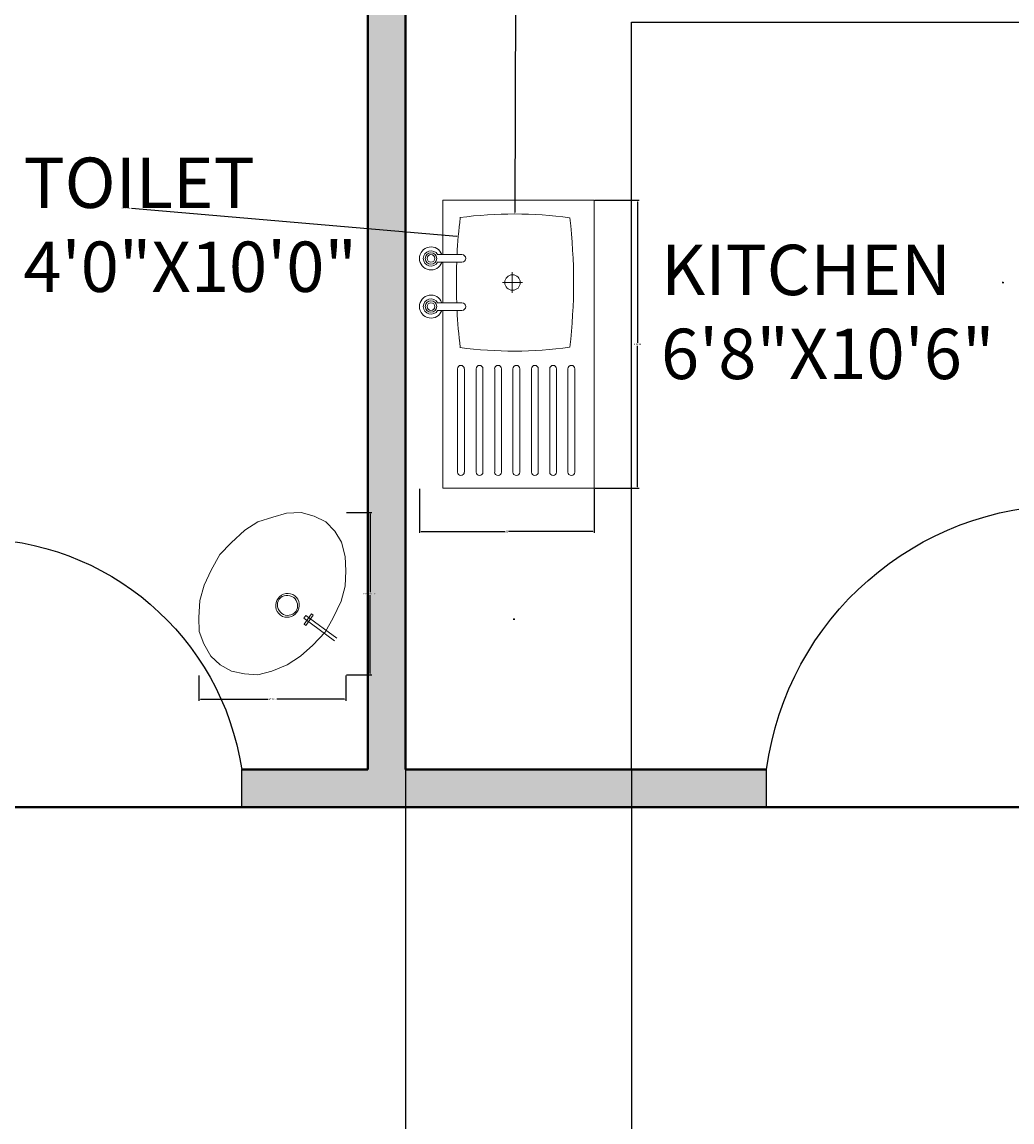
# Model space of a CAD drawing. Units: inches. Extents: x 25176543 to 25177243, y 80295576 to 80296086.
# Tile 7 of 11: x 25176879 to 25176997, y 80295848 to 80295979. Entities that reach past the tile are written whole.
import ezdxf

# ---------------------------------------------------------------- set-up
doc = ezdxf.new("R2010")
doc.units = ezdxf.units.IN
doc.header["$MEASUREMENT"] = 0
for name, color, linetype, lineweight in [('A-ANNO-DIMS', 2, 'Continuous', 18), ('A-AREA-IDEN', 7, 'Continuous', 18), ('A-DOOR', 3, 'Continuous', 25), ('A-FLOR-CASE', 8, 'Continuous', 25), ('A-FLOR-FIXT', 8, 'Continuous', 18), ('A-WALL', 7, 'Continuous', 40), ('A-WALL-PATT', 146, 'Continuous', 13)]:
    doc.layers.add(name, color=color, linetype=linetype, lineweight=lineweight)
doc.styles.get("Standard").update_dxf_attribs({"font": 'arial.ttf'})
doc.dimstyles.get("Standard").update_dxf_attribs({"dimtxt": 0.18, "dimasz": 0.18, "dimexe": 0.18, "dimexo": 0.0625, "dimgap": 0.09, "dimtad": 0, "dimtih": 1, "dimtoh": 1, "dimdec": 4, "dimzin": 0, "dimdsep": 46, "dimtxsty": 'Standard', "dimcen": 0.09, "dimadec": 0, "dimazin": 0, "dimtfac": 1, "dimtdec": 4, "dimtofl": 0, "dimtmove": 0, "dimatfit": 3, "dimfxl": 1, "dimtolj": 1, "dimtzin": 0, "dimarcsym": 0})

# ---------------------------------------------------------------- blocks, each defined once
blk = doc.blocks.new('A$C799204C7')
for p, q in [((0, 34.2), (17.99, 34.2)), ((0, 0), (0, 34.2)), ((17.99, 13.08), (17.99, 34.2)), ((2.32, 20.01), (2.32, 32.27)), ((3.13, 20.01), (3.13, 32.27)), ((4.48, 20.01), (4.48, 32.27)), ((5.29, 20.01), (5.29, 32.27)), ((6.64, 20.01), (6.64, 32.27)), ((7.45, 20.01), (7.45, 32.27)), ((8.85, 20.01), (8.85, 32.27)), ((9.66, 20.01), (9.66, 32.27)), ((11.01, 20.01), (11.01, 32.27)), ((11.82, 20.01), (11.82, 32.27)), ((13.22, 20.01), (13.22, 32.27)), ((14.03, 20.01), (14.03, 32.27)), ((15.42, 20.01), (15.42, 32.27)), ((16.24, 20.01), (16.24, 32.27)), ((18.59, 13.08), (15.71, 13.08)), ((15.71, 12.17), (18.59, 12.17)), ((17.99, 7.36), (17.99, 12.17)), ((9.73, 11), (9.73, 8.54)), ((8.52, 9.77), (10.9, 9.77)), ((18.59, 7.36), (15.71, 7.36)), ((15.71, 6.45), (18.59, 6.45)), ((17.99, 0), (17.99, 6.45)), ((0, 0), (17.99, 0))]:
    blk.add_line(p, q)
for centre, radius in [((19.38, 12.62), 0.684), ((19.38, 12.62), 0.456), ((9.7, 9.77), 0.916), ((19.38, 6.91), 0.684), ((19.38, 6.91), 0.456)]:
    blk.add_circle(centre, radius)
for centre, radius, start, end in [((2.72, 32.27), 0.407, 0, 180), ((4.88, 32.27), 0.407, 0, 180), ((7.05, 32.27), 0.407, 0, 180), ((9.25, 32.27), 0.407, 0, 180), ((11.42, 32.27), 0.407, 0, 180), ((13.62, 32.27), 0.407, 0, 180), ((15.83, 32.27), 0.407, 0, 180), ((2.72, 20.01), 0.407, 180, 0), ((4.88, 20.01), 0.407, 180, 0), ((7.05, 20.01), 0.407, 180, 0), ((9.25, 20.01), 0.407, 180, 0), ((11.42, 20.01), 0.407, 180, 0), ((13.62, 20.01), 0.407, 180, 0), ((15.83, 20.01), 0.407, 180, 0), ((67.33, 9.77), 64.88, 173.1952, 186.8048), ((9.53, -30.19), 48.1, 82.3437, 97.8966), ((-48.51, 9.77), 64.88, 2.9208, 6.8048), ((15.71, 12.62), 0.456, 90, 270), ((19.38, 12.62), 1.37, 199.6514, 160.3603), ((19.38, 12.62), 0.911, 210.3431, 149.7554), ((-48.51, 9.77), 64.88, 357.8723, 2.115), ((19.38, 6.91), 1.37, 199.6514, 160.3603), ((15.71, 6.91), 0.456, 90, 270), ((19.38, 6.91), 0.911, 210.3431, 149.7554), ((-48.51, 9.77), 64.88, 353.1952, 357.0665), ((9.53, 49.73), 48.1, 262.1034, 277.6563)]:
    blk.add_arc(centre, radius, start, end)
blk = doc.blocks.new('WASH-BASIN')
for p, q in [((12.49, 6.73), (12.74, 7.07)), ((13.61, 7.11), (13.41, 7.26)), ((12.71, 5.89), (12.51, 6.04))]:
    blk.add_line(p, q)
for points in [[(2.54, 1.2), (1.42, 2.23), (0.6, 3.68), (0.01, 5.16), (0, 6.84), (0.12, 8.85), (0.63, 10.67), (1.44, 12.48), (2.49, 14.33), (3.84, 15.74), (5.48, 17.25), (7.03, 18.21), (8.81, 18.78), (10.43, 19.26), (12.16, 19.34), (13.73, 18.91), (15.1, 18.22), (16.17, 17.11), (16.98, 15.79), (17.41, 14.1), (17.49, 12.37), (17.4, 10.55), (16.94, 8.79), (15.98, 6.78), (15.03, 5.07), (13.58, 3.52), (12.09, 2.21), (10.49, 1.19), (8.68, 0.43), (7, 0), (5.41, 0.12), (3.86, 0.43)], [(12.59, 6.87), (12.59, 6.87)], [(13.33, 7.16), (13.33, 7.16)], [(12.43, 5.94), (12.43, 5.94)]]:
    blk.add_lwpolyline(points, close=True)
for points in [[(16.15, 4.03), (12.49, 6.73), (12.49, 6.73)], [(12.51, 6.04), (13.41, 7.26), (13.41, 7.26)], [(12.71, 5.89), (13.61, 7.11), (13.61, 7.11)], [(16.4, 4.37), (12.74, 7.07), (12.74, 7.07)]]:
    blk.add_lwpolyline(points)
for points in [[(9.72, 7.1), (10.34, 6.65), (11.21, 6.84), (11.66, 7.45), (11.66, 7.45), (12.11, 8.06), (12.04, 8.96), (11.43, 9.41), (11.43, 9.41), (10.75, 9.91), (9.87, 9.71), (9.42, 9.1), (9.42, 9.1), (8.97, 8.49), (9.05, 7.6), (9.72, 7.1)], [(9.88, 7.3), (10.35, 6.95), (11.12, 7.01), (11.53, 7.55), (11.53, 7.55), (11.93, 8.1), (11.75, 8.85), (11.28, 9.2), (11.28, 9.2), (10.73, 9.6), (9.96, 9.55), (9.56, 9), (9.56, 9), (9.16, 8.46), (9.33, 7.7), (9.88, 7.3)]]:
    blk.add_open_spline(points, degree=3, knots=[0, 0, 0, 0, 0.0625, 0.0625, 0.0625, 0.062501, 0.125, 0.125, 0.125, 0.125001, 0.1875, 0.1875, 0.1875, 0.187501, 1, 1, 1, 1])
blk = doc.blocks.new('DOOR-32IN')
for p, q in [((0, 1), (0, 33)), ((0, 33), (4.5, 33)), ((32, 2), (0, 2)), ((0, 0), (0, 1)), ((0, 1), (32, 1)), ((32, 1), (0, 1))]:
    blk.add_line(p, q)
blk.add_arc((-0.37, 1), 32.37, 0, 81.3499)
blk = doc.blocks.new('DOOR-36IN')
for p, q in [((36, 37), (31.5, 37)), ((36, 1), (36, 37)), ((0, 2), (36, 2)), ((36, 1), (0, 1)), ((0, 1), (36, 1)), ((36, 0), (36, 1))]:
    blk.add_line(p, q)
blk.add_arc((36.32, 1), 36.32, 97.6281, 180)
blk = doc.blocks.new('*D32')
at = {"layer": 'A-ANNO-DIMS', "color": 0, "lineweight": -2, "transparency": 16777216}
for p, q in [((25176917.26, 80295920.91), (25176920.28, 80295920.91)), ((25176920.1, 80295920.73), (25176920.1, 80295911.42)), ((25176920.1, 80295901.74), (25176920.1, 80295911.05)), ((25176917.26, 80295901.56), (25176920.28, 80295901.56))]:
    blk.add_line(p, q, dxfattribs=at)
at = {"layer": 'A-ANNO-DIMS', "color": 0, "transparency": 16777216}
for points in [[(25176920.07, 80295920.73), (25176920.13, 80295920.73), (25176920.1, 80295920.91)], [(25176920.07, 80295901.74), (25176920.13, 80295901.74), (25176920.1, 80295901.56)]]:
    blk.add_solid(points, dxfattribs=at)
at = {"layer": 'Defpoints', "color": 0, "transparency": 16777216}
for p in [(25176917.2, 80295920.91), (25176920.1, 80295920.91), (25176917.2, 80295901.56)]:
    blk.add_point(p, dxfattribs=at)
at = {"layer": 'A-ANNO-DIMS', "color": 0, "transparency": 16777216, "insert": (25176920.1, 80295911.23), "char_height": 0.18, "attachment_point": 5}
blk.add_mtext('\\A1;BASIN 19 TYP.', dxfattribs=at)
blk = doc.blocks.new('*D33')
at = {"layer": 'A-ANNO-DIMS', "color": 0, "lineweight": -2, "transparency": 16777216}
for p, q in [((25176899.71, 80295901.5), (25176899.71, 80295898.48)), ((25176917.2, 80295901.5), (25176917.2, 80295898.48)), ((25176899.89, 80295898.66), (25176907.93, 80295898.66)), ((25176917.02, 80295898.66), (25176908.97, 80295898.66))]:
    blk.add_line(p, q, dxfattribs=at)
at = {"layer": 'A-ANNO-DIMS', "color": 0, "transparency": 16777216}
for points in [[(25176899.89, 80295898.69), (25176899.89, 80295898.63), (25176899.71, 80295898.66)], [(25176917.02, 80295898.69), (25176917.02, 80295898.63), (25176917.2, 80295898.66)]]:
    blk.add_solid(points, dxfattribs=at)
at = {"layer": 'Defpoints', "color": 0, "transparency": 16777216}
for p in [(25176899.71, 80295901.56), (25176917.2, 80295901.56), (25176917.2, 80295898.66)]:
    blk.add_point(p, dxfattribs=at)
at = {"layer": 'A-ANNO-DIMS', "color": 0, "transparency": 16777216, "insert": (25176908.45, 80295898.66), "char_height": 0.18, "attachment_point": 5}
blk.add_mtext('\\A1;17 TYP.', dxfattribs=at)
blk = doc.blocks.new('*D44')
at = {"layer": 'A-ANNO-DIMS', "color": 0, "lineweight": -2, "transparency": 16777216}
for p, q in [((25176946.84, 80295958.09), (25176952.11, 80295958.09)), ((25176951.93, 80295957.91), (25176951.93, 80295941.12)), ((25176951.93, 80295923.96), (25176951.93, 80295940.75)), ((25176946.84, 80295923.78), (25176952.11, 80295923.78))]:
    blk.add_line(p, q, dxfattribs=at)
at = {"layer": 'A-ANNO-DIMS', "color": 0, "transparency": 16777216}
for points in [[(25176951.9, 80295957.91), (25176951.96, 80295957.91), (25176951.93, 80295958.09)], [(25176951.9, 80295923.96), (25176951.96, 80295923.96), (25176951.93, 80295923.78)]]:
    blk.add_solid(points, dxfattribs=at)
at = {"layer": 'Defpoints', "color": 0, "transparency": 16777216}
for p in [(25176946.78, 80295958.09), (25176946.78, 80295923.78), (25176951.93, 80295923.78)]:
    blk.add_point(p, dxfattribs=at)
at = {"layer": 'A-ANNO-DIMS', "color": 0, "transparency": 16777216, "insert": (25176951.93, 80295940.94), "char_height": 0.18, "attachment_point": 5}
blk.add_mtext('\\A1;SINK 34', dxfattribs=at)
blk = doc.blocks.new('*D45')
at = {"layer": 'A-ANNO-DIMS', "color": 0, "lineweight": -2, "transparency": 16777216}
for p, q in [((25176925.97, 80295923.72), (25176925.97, 80295918.46)), ((25176946.78, 80295923.72), (25176946.78, 80295918.46)), ((25176926.15, 80295918.64), (25176936.17, 80295918.64)), ((25176946.6, 80295918.64), (25176936.58, 80295918.64))]:
    blk.add_line(p, q, dxfattribs=at)
at = {"layer": 'A-ANNO-DIMS', "color": 0, "transparency": 16777216}
for points in [[(25176926.15, 80295918.67), (25176926.15, 80295918.61), (25176925.97, 80295918.64)], [(25176946.6, 80295918.67), (25176946.6, 80295918.61), (25176946.78, 80295918.64)]]:
    blk.add_solid(points, dxfattribs=at)
at = {"layer": 'Defpoints', "color": 0, "transparency": 16777216}
for p in [(25176925.97, 80295923.78), (25176946.78, 80295923.78), (25176925.97, 80295918.64)]:
    blk.add_point(p, dxfattribs=at)
at = {"layer": 'A-ANNO-DIMS', "color": 0, "transparency": 16777216, "insert": (25176936.37, 80295918.64), "char_height": 0.18, "attachment_point": 5}
blk.add_mtext('\\A1;21', dxfattribs=at)
blk = doc.blocks.new('*D48')
at = {"layer": 'A-ANNO-DIMS', "color": 0, "lineweight": -2, "transparency": 16777216}
for p, q in [((25176625.3, 80295890.36), (25176625.3, 80296052.23)), ((25176625.48, 80296052.05), (25176875.16, 80296052.05)), ((25177125.62, 80296052.05), (25176875.95, 80296052.05)), ((25177125.8, 80296025.36), (25177125.8, 80296052.23))]:
    blk.add_line(p, q, dxfattribs=at)
at = {"layer": 'A-ANNO-DIMS', "color": 0, "transparency": 16777216}
for points in [[(25176625.48, 80296052.08), (25176625.48, 80296052.02), (25176625.3, 80296052.05)], [(25177125.62, 80296052.08), (25177125.62, 80296052.02), (25177125.8, 80296052.05)]]:
    blk.add_solid(points, dxfattribs=at)
at = {"layer": 'Defpoints', "color": 0, "transparency": 16777216}
for p in [(25177125.8, 80296052.05), (25177125.8, 80296025.3), (25176625.3, 80295890.3)]:
    blk.add_point(p, dxfattribs=at)
at = {"layer": 'A-ANNO-DIMS', "color": 0, "transparency": 16777216, "insert": (25176875.55, 80296052.05), "char_height": 0.18, "attachment_point": 5}
blk.add_mtext('\\A1;500.5', dxfattribs=at)
blk = doc.blocks.new('*D69')
at = {"layer": 'A-ANNO-DIMS', "color": 0, "lineweight": -2, "transparency": 16777216}
for p, q in [((25176924.3, 80295890.24), (25176924.3, 80295640.87)), ((25176951.22, 80295890.24), (25176951.22, 80295640.87)), ((25176924.48, 80295641.05), (25176937.37, 80295641.05)), ((25176951.04, 80295641.05), (25176938.16, 80295641.05))]:
    blk.add_line(p, q, dxfattribs=at)
at = {"layer": 'A-ANNO-DIMS', "color": 0, "transparency": 16777216}
for points in [[(25176924.48, 80295641.08), (25176924.48, 80295641.02), (25176924.3, 80295641.05)], [(25176951.04, 80295641.08), (25176951.04, 80295641.02), (25176951.22, 80295641.05)]]:
    blk.add_solid(points, dxfattribs=at)
at = {"layer": 'Defpoints', "color": 0, "transparency": 16777216}
for p in [(25176924.3, 80295890.3), (25176951.22, 80295890.3), (25176951.22, 80295641.05)]:
    blk.add_point(p, dxfattribs=at)
at = {"layer": 'A-ANNO-DIMS', "color": 0, "transparency": 16777216, "insert": (25176937.76, 80295641.05), "char_height": 0.18, "attachment_point": 5}
blk.add_mtext('\\A1;26.92', dxfattribs=at)
blk = doc.blocks.new('*D78')
at = {"layer": 'A-ANNO-DIMS', "color": 0, "lineweight": -2, "transparency": 16777216}
for p, q in [((25176891.69, 80295957.13), (25176930.42, 80295953.83)), ((25176995.36, 80295948.29), (25176995.54, 80295948.29)), ((25176995.45, 80295948.2), (25176995.45, 80295948.38))]:
    blk.add_line(p, q, dxfattribs=at)
at = {"layer": 'A-ANNO-DIMS', "color": 0, "transparency": 16777216}
blk.add_solid([(25176930.42, 80295953.86), (25176930.42, 80295953.8), (25176930.6, 80295953.81)], dxfattribs=at)
at = {"layer": 'Defpoints', "color": 0, "transparency": 16777216}
for p in [(25176930.6, 80295953.81), (25176995.45, 80295948.29)]:
    blk.add_point(p, dxfattribs=at)
at = {"layer": 'A-ANNO-DIMS', "color": 0, "transparency": 16777216, "insert": (25176891.01, 80295957.13), "char_height": 0.18, "attachment_point": 5}
blk.add_mtext('\\A1;4X R65.08', dxfattribs=at)
blk = doc.blocks.new('*D79')
at = {"layer": 'A-ANNO-DIMS', "color": 0, "lineweight": -2, "transparency": 16777216}
for p, q in [((25176937.39, 80295985.41), (25176937.33, 80295956.64)), ((25176937.57, 80295985.41), (25176937.39, 80295985.41)), ((25176937.14, 80295908.2), (25176937.32, 80295908.2)), ((25176937.23, 80295908.11), (25176937.23, 80295908.29))]:
    blk.add_line(p, q, dxfattribs=at)
at = {"layer": 'A-ANNO-DIMS', "color": 0, "transparency": 16777216}
blk.add_solid([(25176937.3, 80295956.64), (25176937.36, 80295956.64), (25176937.33, 80295956.46)], dxfattribs=at)
at = {"layer": 'Defpoints', "color": 0, "transparency": 16777216}
for p in [(25176937.33, 80295956.46), (25176937.23, 80295908.2)]:
    blk.add_point(p, dxfattribs=at)
at = {"layer": 'A-ANNO-DIMS', "color": 0, "transparency": 16777216, "insert": (25176938.24, 80295985.41), "char_height": 0.18, "attachment_point": 5}
blk.add_mtext('\\A1;2X R48.26', dxfattribs=at)

msp = doc.modelspace()

# ---------------------------------------------------------------- hatches: boundary and pattern name
at = {"layer": 'A-WALL-PATT'}
h = msp.add_hatch(color=256, dxfattribs=at)
h.dxf.hatch_style = 1
h.paths.add_polyline_path([(25176695.189, 80296025.3022), (25176658.8016, 80296025.3022), (25176658.8016, 80296016.3022), (25176695.189, 80296016.3022)])
h.paths.add_polyline_path([(25176810.3016, 80296025.3022), (25176755.189, 80296025.3022), (25176755.189, 80296016.3022), (25176810.3016, 80296016.3022)])
h.paths.add_polyline_path([(25176819.3016, 80296016.3022), (25176814.8016, 80296016.3022), (25176814.8016, 80295965.3022), (25176819.3016, 80295965.3022)], flags=17)
h.paths.add_polyline_path([(25176828.0421, 80296025.3022), (25176819.3016, 80296025.3022), (25176819.3016, 80296016.3022), (25176828.0421, 80296016.3022)])
h.paths.add_polyline_path([(25176867.3016, 80296025.3022), (25176852.0421, 80296025.3022), (25176852.0421, 80296016.3022), (25176867.3016, 80296016.3022)])
h.paths.add_polyline_path([(25176885.1873, 80296025.3022), (25176876.3016, 80296025.3022), (25176876.3016, 80296016.3022), (25176885.1873, 80296016.3022)])
h.paths.add_polyline_path([(25176919.8016, 80296025.3022), (25176909.1873, 80296025.3022), (25176909.1873, 80296016.3022), (25176919.8016, 80296016.3022)])
h.paths.add_polyline_path([(25176924.3016, 80296016.3022), (25176919.8016, 80296016.3022), (25176919.8016, 80295890.3022), (25176904.8016, 80295890.3022), (25176904.8016, 80295885.8022), (25176967.3016, 80295885.8022), (25176967.3016, 80295890.3022), (25176924.3016, 80295890.3022)])
h.paths.add_polyline_path([(25176924.3016, 80296025.3022), (25176919.8016, 80296025.3022), (25176919.8016, 80296016.3022), (25176924.3016, 80296016.3022)])
h.paths.add_polyline_path([(25176938.7147, 80296025.3022), (25176924.3016, 80296025.3022), (25176924.3016, 80296016.3022), (25176938.7147, 80296016.3022)])
h.paths.add_polyline_path([(25176871.8016, 80296016.3022), (25176867.3016, 80296016.3022), (25176867.3016, 80295932.3022), (25176819.3016, 80295932.3022), (25176819.3016, 80295933.3022), (25176814.8016, 80295933.3022), (25176814.8016, 80295932.3022), (25176814.8016, 80295927.3022), (25176819.3016, 80295927.3022), (25176819.3016, 80295927.8022), (25176867.3016, 80295927.8022), (25176867.3016, 80295885.8022), (25176871.8016, 80295885.8022), (25176872.8016, 80295885.8022), (25176872.8016, 80295890.3022), (25176871.8016, 80295890.3022)])
h.paths.add_polyline_path([(25177004.3016, 80296025.3022), (25176986.7147, 80296025.3022), (25176986.7147, 80296016.3022), (25177004.3016, 80296016.3022)])
h.paths.add_polyline_path([(25177035.845, 80296025.3022), (25177013.3016, 80296025.3022), (25177013.3016, 80296016.3022), (25177035.845, 80296016.3022)])
h.paths.add_polyline_path([(25177008.8016, 80296016.3022), (25177004.3016, 80296016.3022), (25177004.3016, 80295890.3022), (25177003.3016, 80295890.3022), (25177003.3016, 80295885.8022), (25177004.3016, 80295885.8022), (25177004.3016, 80295885.3022), (25177008.8016, 80295885.3022)])
h.paths.add_polyline_path([(25177116.8016, 80296025.3022), (25177095.845, 80296025.3022), (25177095.845, 80296016.3022), (25177116.8016, 80296016.3022)])
h.paths.add_polyline_path([(25177125.8016, 80296016.3022), (25177116.8016, 80296016.3022), (25177116.8016, 80295971.1334), (25177121.3016, 80295971.1334), (25177125.8016, 80295971.1334)])
h.paths.add_polyline_path([(25177116.8016, 80295848.3022), (25177013.3016, 80295848.3022), (25177013.3016, 80295843.8022), (25177116.8016, 80295843.8022)])
h.paths.add_polyline_path([(25177125.8016, 80295911.1334), (25177116.8016, 80295911.1334), (25177116.8016, 80295848.3022), (25177125.8016, 80295848.3022)])
h.paths.add_polyline_path([(25177008.8016, 80295802.3022), (25177004.3016, 80295802.3022), (25177004.3016, 80295676.8022), (25177008.8016, 80295676.8022)])
h.paths.add_polyline_path([(25176658.8016, 80295705.5694), (25176649.8016, 80295705.5694), (25176649.8016, 80295676.8022), (25176658.8016, 80295676.8022)])
h.paths.add_polyline_path([(25176658.8016, 80295798.3022), (25176649.8016, 80295798.3022), (25176649.8016, 80295765.5694), (25176654.3016, 80295765.5694), (25176658.8016, 80295765.5694)])
h.paths.add_polyline_path([(25176833.3016, 80295807.3022), (25176658.8016, 80295807.3022), (25176658.8016, 80295802.8022), (25176833.3016, 80295802.8022)])
h.paths.add_polyline_path([(25176842.3016, 80295761.3022), (25176837.8016, 80295761.3022), (25176837.8016, 80295676.8022), (25176842.3016, 80295676.8022)])
h.paths.add_polyline_path([(25176649.8016, 80295807.3022), (25176629.8016, 80295807.3022), (25176629.8016, 80295885.8022), (25176649.8016, 80295885.8022), (25176649.8016, 80295890.3022), (25176625.3016, 80295890.3022), (25176625.3016, 80295802.8022), (25176649.8016, 80295802.8022)])
h.paths.add_polyline_path([(25176810.3016, 80295890.3022), (25176658.8016, 80295890.3022), (25176658.8016, 80295885.8022), (25176810.3016, 80295885.8022)])
h.paths.add_polyline_path([(25176658.8016, 80295922.9263), (25176649.8016, 80295922.9263), (25176649.8016, 80295890.3022), (25176658.8016, 80295890.3022)])
h.paths.add_polyline_path([(25176658.8016, 80296016.3022), (25176649.8016, 80296016.3022), (25176649.8016, 80295982.9263), (25176654.3016, 80295982.9263), (25176658.8016, 80295982.9263)])

# ---------------------------------------------------------------- linework, layer by layer
at = {"layer": 'A-FLOR-CASE'}
for p, q in [((25176951.2221, 80295890.3022), (25176951.2221, 80295979.3235)), ((25176951.2221, 80295979.3235), (25177004.3016, 80295979.3235)), ((25176951.2221, 80295890.3022), (25176951.2221, 80295890.3022))]:
    msp.add_line(p, q, dxfattribs=at)
at = {"layer": 'A-WALL'}
for p, q in [((25176919.8016, 80296025.3022), (25176919.8016, 80295890.3022)), ((25176924.3016, 80296025.3022), (25176924.3016, 80295890.3022)), ((25176904.8016, 80295890.3022), (25176919.8016, 80295890.3022)), ((25176924.3016, 80295890.3022), (25176967.3016, 80295890.3022)), ((25176867.3016, 80295885.8022), (25177004.3016, 80295885.8022)), ((25176924.3016, 80295885.8022), (25176925.3016, 80295885.8022))]:
    msp.add_line(p, q, dxfattribs=at)

# ---------------------------------------------------------------- block references
at = {"layer": 'A-DOOR', "extrusion": (0, 0, -1), "zscale": -1}
for name, p, rotation in [('DOOR-36IN', (-25177004.3018, 80295921.8018), 270.0000000097776), ('DOOR-32IN', (-25176871.8014, 80295885.8026), 90.00000000616691)]:
    msp.add_blockref(name, p, dxfattribs=dict(at, rotation=rotation))
at = {"layer": 'A-FLOR-FIXT', "xscale": 1.0032, "yscale": 1.0032, "zscale": 1.0032, "rotation": 180}
msp.add_blockref('A$C799204C7', (25176946.7808, 80295958.0909), dxfattribs=at)
at = {"layer": 'A-FLOR-FIXT'}
msp.add_blockref('WASH-BASIN', (25176899.7068, 80295901.5643), dxfattribs=at)

# ---------------------------------------------------------------- texts
at = {"layer": 'A-AREA-IDEN', "char_height": 6, "attachment_point": 1}
for s, width, insert in [('TOILET\\P4\'0"X10\'0"', 34.433499, (25176878.8103, 80295963.173)), ('KITCHEN\\P6\'8"X10\'6"', 49.577747, (25176954.7238, 80295952.7922))]:
    msp.add_mtext_dynamic_manual_height_columns(s, width=width, gutter_width=1, heights=[0], dxfattribs=dict(at, insert=insert))

# ---------------------------------------------------------------- dimensions: what is measured, and where the dimension line sits
at = {"layer": 'A-ANNO-DIMS'}
for base, p1, p2, override, picture, middle in [((25177125.8016, 80296052.0522), (25176625.3016, 80295890.3022), (25177125.8016, 80296025.3022), {"dimdec": 1, "dimlfac": 1, "dimrnd": 0, "dimzin": 0, "dimdsep": 46, "dimlunit": 2}, '*D48', (25176875.5516, 80296052.0522)), ((25176951.2221, 80295641.0522), (25176924.3016, 80295890.3022), (25176951.2221, 80295890.3022), {"dimdec": 2, "dimlfac": 1, "dimrnd": 0, "dimzin": 0, "dimdsep": 46, "dimlunit": 2}, '*D69', (25176937.7618, 80295641.0522))]:
    dim = msp.add_linear_dim(base=base, p1=p1, p2=p2, dimstyle='Standard', override=override, dxfattribs=at)
    dim.commit()
    dim.dimension.update_dxf_attribs({"geometry": picture, "text_midpoint": middle})
for center, mpoint, text, picture, middle in [((25176937.225, 80295908.2018), (25176937.326, 80295956.4572), '2X <>', '*D79', (25176938.2413, 80295985.4104)), ((25176995.4478, 80295948.2882), (25176930.5999, 80295953.812), '4X <>', '*D78', (25176891.6912, 80295957.1263))]:
    dim = msp.add_radius_dim(center=center, mpoint=mpoint, text=text, dimstyle='Standard', override={"dimdec": 2, "dimlfac": 1, "dimrnd": 0, "dimzin": 0, "dimdsep": 46, "dimlunit": 2}, dxfattribs=at)
    dim.commit()
    dim.dimension.update_dxf_attribs({"geometry": picture, "text_midpoint": middle, "dimtype": 164})
for base, p1, p2, angle, text, picture, middle in [((25176951.9272, 80295923.7815), (25176946.7808, 80295958.0909), (25176946.7808, 80295923.7815), 270, 'SINK <>', '*D44', (25176951.9272, 80295940.9362)), ((25176920.0981, 80295920.9053), (25176917.197, 80295901.5644), (25176917.197, 80295920.9053), 90, 'BASIN <> TYP.', '*D32', (25176920.0981, 80295911.2349))]:
    dim = msp.add_linear_dim(base=base, p1=p1, p2=p2, angle=angle, text=text, dimstyle='Standard', override={"dimdec": 0, "dimlfac": 1, "dimrnd": 0, "dimzin": 0, "dimdsep": 46, "dimlunit": 2}, dxfattribs=at)
    dim.commit()
    dim.dimension.update_dxf_attribs({"geometry": picture, "text_midpoint": middle})
dim = msp.add_linear_dim(base=(25176925.9668, 80295918.6351), p1=(25176946.7808, 80295923.7815), p2=(25176925.9668, 80295923.7815), angle=180, dimstyle='Standard', override={"dimdec": 0, "dimlfac": 1, "dimrnd": 0, "dimzin": 0, "dimdsep": 46, "dimlunit": 2}, dxfattribs=at)
dim.commit()
dim.dimension.update_dxf_attribs({"geometry": '*D45', "text_midpoint": (25176936.3738, 80295918.6351)})
dim = msp.add_linear_dim(base=(25176917.197, 80295898.6633), p1=(25176899.7067, 80295901.5644), p2=(25176917.197, 80295901.5644), text='<> TYP.', dimstyle='Standard', override={"dimdec": 0, "dimlfac": 1, "dimrnd": 0, "dimzin": 0, "dimdsep": 46, "dimlunit": 2}, dxfattribs=at)
dim.commit()
dim.dimension.update_dxf_attribs({"geometry": '*D33', "text_midpoint": (25176908.4519, 80295898.6633)})

doc.saveas('drawing.dxf')
